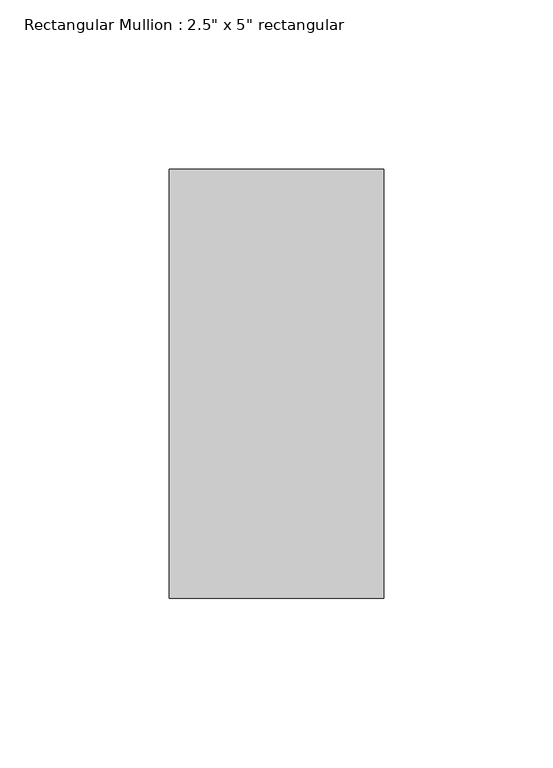
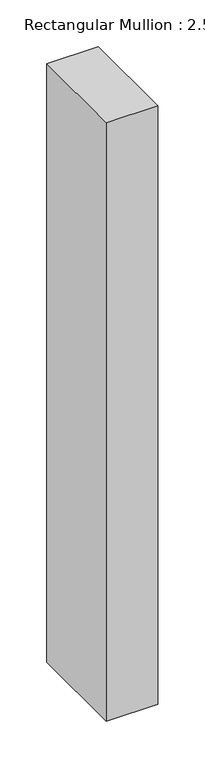
"""IFC4 building model written with IfcOpenShell, lengths in millimetres: member geometry."""

from ifc_helpers import new_model, si_unit, frame, origin, place, context, project, spatial, polyline, outline, extrude, source, transform, mapped, element, save


def member_6d419de8(model_context):
    return source(origin(), model_context, "Body", "SweptSolid", [
        extrude(outline(polyline([(0.0, 63.5), (0.0, -63.5), (-63.5, -63.5), (-63.5, 63.5), (0.0, 63.5)])), frame((0.0, 0.0, -779.9323007), z_axis=(0.0, 0.0, 1.0), x_axis=(1.0, 0.0, 0.0)), (0.0, 0.0, 1.0), 779.9323007),
    ])


if __name__ == "__main__":
    model = new_model("IFC4")
    model_context = context("Model", 3, world=origin())
    ifc_project = project(units=[si_unit("LENGTHUNIT", "METRE", prefix="MILLI")], contexts=[model_context])
    site = spatial("IfcSite", under=ifc_project)
    building = spatial("IfcBuilding", under=site)
    placement = place(None, origin())
    member_shape = member_6d419de8(model_context)
    element("IfcMember", 1, ObjectType="Rectangular Mullion : 2.5\" x 5\" rectangular", at=placement, inside=building, context=model_context, shape_type="MappedRepresentation", body=[
        mapped(member_shape, transform((0.0, 0.0, 0.0), x_axis=(1.0, 0.0, 0.0), y_axis=(0.0, 1.0, 0.0), z_axis=(0.0, 0.0, 1.0))),
    ])
    save(model, "model.ifc")

# Revit data of these elements
# Type "Rectangular Mullion : 2.5\" x 5\" rectangular"
#   built-in parameter 1007304 = 0.416667 (stored number, unit not read)
#   built-in parameter 1007301 = 0.104167 (stored number, unit not read)
#   built-in parameter 1007300 = 0.104167 (stored number, unit not read)
# Element 1 (IfcMember, "Rectangular Mullion : 2.5\" x 5\" rectangular")
#   Materials on its faces: "Aluminum"
# Materials
#   "Aluminum": class "Metal", colour RGB 247 247 247, transparency 0, Description = "Aluminum 6061", Cost = 0
